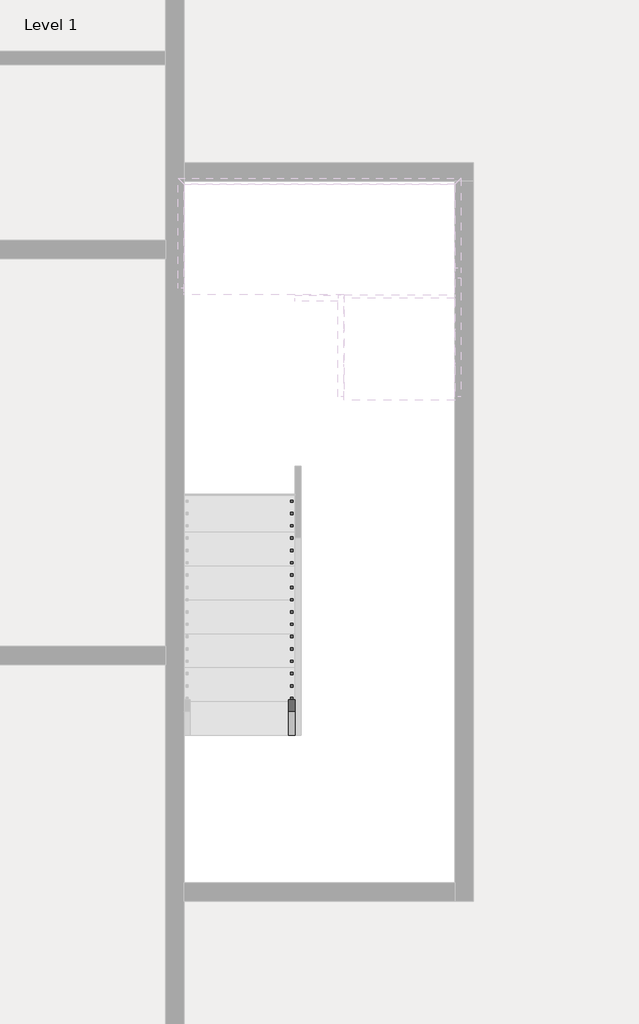
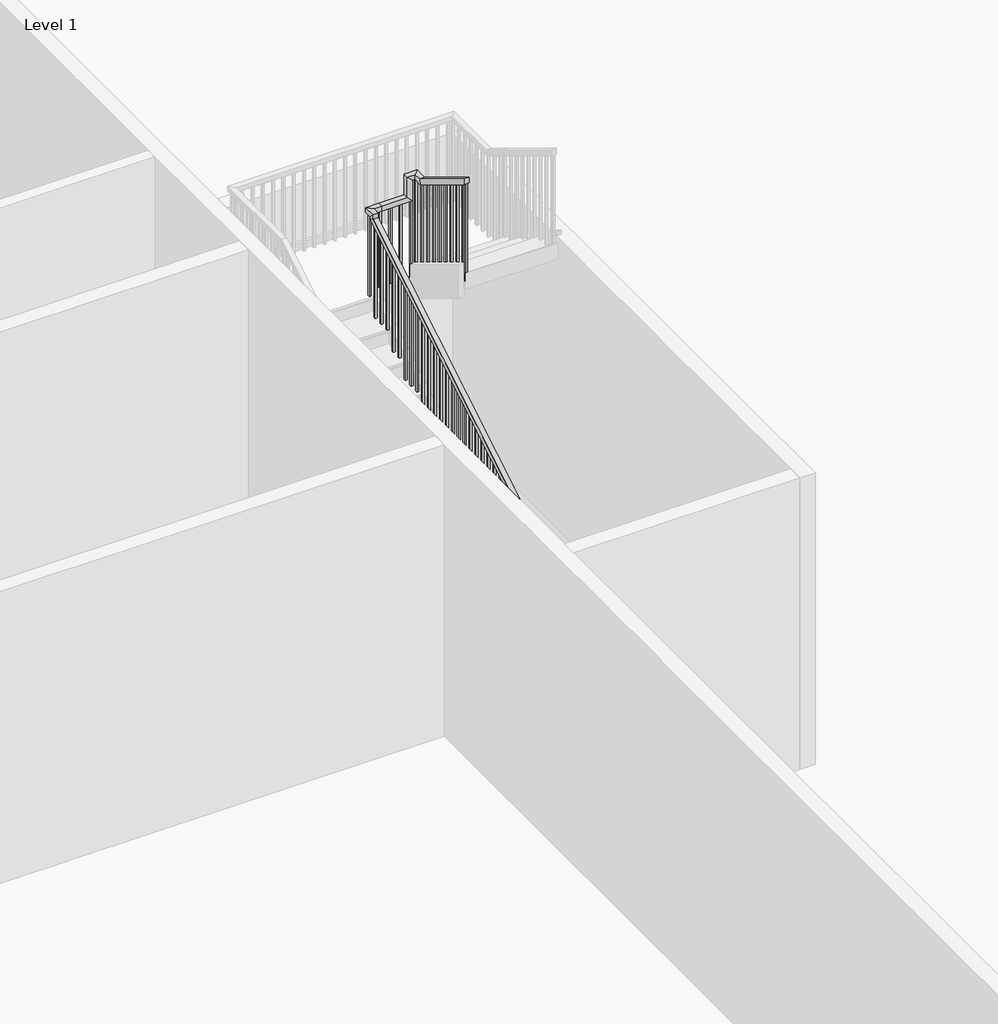
# One storey, part 5 of 8: 1 railing.
"""IFC4 building model written with IfcOpenShell, lengths in millimetres."""

from ifc_helpers import new_model, si_unit, frame, origin, place, context, project, spatial, polyline, outline, extrude, faceted_brep, element, save

model = new_model("IFC4")

# Units and contexts
model_context = context("Model", 3, world=origin())
ifc_project = project(units=[si_unit("LENGTHUNIT", "METRE", prefix="MILLI")], contexts=[model_context])

# Site, building, storey
site = spatial("IfcSite", under=ifc_project)
building = spatial("IfcBuilding", under=site)
storey = spatial("IfcBuildingStorey", under=building, Name="Level 1", Elevation=25234.6172466)

# Railing
placement = place(None, origin())
element("IfcRailing", 1, ObjectType="Handrail - Rectangular", at=placement, inside=storey, context=model_context, shape_type="SolidModel", body=[
    faceted_brep([(-2753.8415084, -23154.3851539, 26318.3505799), (-2753.8415084, -23154.3851539, 26258.9491197), (-2703.0415084, -23154.3851539, 26258.9491197), (-2703.0415084, -23154.3851539, 26318.3505799), (-2753.8415084, -19598.3851539, 28473.5020951), (-2753.8415084, -19547.5851539, 28444.8885136), (-2703.0415084, -19547.5851539, 28444.8885136), (-2703.0415084, -19598.3851539, 28473.5020951), (-2753.8415084, -19598.3851539, 28519.6839133), (-2753.8415084, -19547.5851539, 28468.8839133), (-2703.0415084, -19547.5851539, 28468.8839133), (-2703.0415084, -19598.3851539, 28519.6839133), (-2753.8415084, -19471.3851539, 28519.6839133), (-2753.8415084, -19471.3851539, 28468.8839133), (-2703.0415084, -19522.1851539, 28468.8839133), (-2703.0415084, -19522.1851539, 28519.6839133), (-2626.8415084, -19471.3851539, 28519.6839133), (-2626.8415084, -19471.3851539, 28468.8839133), (-2626.8415084, -19522.1851539, 28468.8839133), (-2626.8415084, -19522.1851539, 28519.6839133), (-2372.8415084, -19471.3851539, 28519.6839133), (-2322.0415084, -19471.3851539, 28468.8839133), (-2322.0415084, -19522.1851539, 28468.8839133), (-2372.8415084, -19522.1851539, 28519.6839133), (-2372.8415084, -19471.3851539, 28735.1990648), (-2322.0415084, -19471.3851539, 28684.3990648), (-2322.0415084, -19522.1851539, 28684.3990648), (-2372.8415084, -19522.1851539, 28735.1990648), (-2245.8415084, -19471.3851539, 28735.1990648), (-2245.8415084, -19471.3851539, 28684.3990648), (-2296.6415084, -19522.1851539, 28684.3990648), (-2296.6415084, -19522.1851539, 28735.1990648), (-2245.8415084, -19598.3851539, 28735.1990648), (-2245.8415084, -19612.5775633, 28684.3990648), (-2296.6415084, -19612.5775633, 28684.3990648), (-2296.6415084, -19598.3851539, 28735.1990648), (-2245.8415084, -20360.3851539, 29197.0172466), (-2296.6415084, -20360.3851539, 29197.0172466), (-2296.6415084, -20360.3851539, 29137.6157863), (-2245.8415084, -20360.3851539, 29137.6157863)], [[[0, 1, 2, 3]], [[1, 0, 4, 5]], [[2, 1, 5, 6]], [[3, 2, 6, 7]], [[0, 3, 7, 4]], [[5, 4, 8, 9]], [[6, 5, 9, 10]], [[7, 6, 10, 11]], [[4, 7, 11, 8]], [[9, 8, 12, 13]], [[10, 9, 13, 14]], [[11, 10, 14, 15]], [[8, 11, 15, 12]], [[13, 12, 16, 17]], [[14, 13, 17, 18]], [[15, 14, 18, 19]], [[12, 15, 19, 16]], [[17, 16, 20, 21]], [[18, 17, 21, 22]], [[19, 18, 22, 23]], [[16, 19, 23, 20]], [[21, 20, 24, 25]], [[22, 21, 25, 26]], [[23, 22, 26, 27]], [[20, 23, 27, 24]], [[25, 24, 28, 29]], [[26, 25, 29, 30]], [[27, 26, 30, 31]], [[24, 27, 31, 28]], [[29, 28, 32, 33]], [[30, 29, 33, 34]], [[31, 30, 34, 35]], [[28, 31, 35, 32]], [[36, 37, 38, 39]], [[33, 32, 36, 39]], [[34, 33, 39, 38]], [[35, 34, 38, 37]], [[32, 35, 37, 36]]]),
    extrude(outline(polyline([(-20319.1101539, 29112.6006348), (-20300.0601539, 29101.0551803), (-20300.0601539, 28113.2839133), (-20319.1101539, 28113.2839133), (-20319.1101539, 29112.6006348)])), frame((-2280.7665084, 0.0, 0.0), z_axis=(1.0, 0.0, 0.0), x_axis=(0.0, 1.0, 0.0)), (0.0, 0.0, 1.0), 19.05),
    extrude(outline(polyline([(-20217.5101539, 29051.0248773), (-20198.4601539, 29039.4794227), (-20198.4601539, 28113.2839133), (-20217.5101539, 28113.2839133), (-20217.5101539, 29051.0248773)])), frame((-2280.7665084, 0.0, 0.0), z_axis=(1.0, 0.0, 0.0), x_axis=(0.0, 1.0, 0.0)), (0.0, 0.0, 1.0), 19.05),
    extrude(outline(polyline([(-20115.9101539, 28989.4491197), (-20096.8601539, 28977.9036651), (-20096.8601539, 28113.2839133), (-20115.9101539, 28113.2839133), (-20115.9101539, 28989.4491197)])), frame((-2280.7665084, 0.0, 0.0), z_axis=(1.0, 0.0, 0.0), x_axis=(0.0, 1.0, 0.0)), (0.0, 0.0, 1.0), 19.05),
    extrude(outline(polyline([(-20014.3101539, 28927.8733621), (-19995.2601539, 28916.3279076), (-19995.2601539, 27943.9505799), (-20014.3101539, 27943.9505799), (-20014.3101539, 28927.8733621)])), frame((-2280.7665084, 0.0, 0.0), z_axis=(1.0, 0.0, 0.0), x_axis=(0.0, 1.0, 0.0)), (0.0, 0.0, 1.0), 19.05),
    extrude(outline(polyline([(-19912.7101539, 28866.2976045), (-19893.6601539, 28854.75215), (-19893.6601539, 27943.9505799), (-19912.7101539, 27943.9505799), (-19912.7101539, 28866.2976045)])), frame((-2280.7665084, 0.0, 0.0), z_axis=(1.0, 0.0, 0.0), x_axis=(0.0, 1.0, 0.0)), (0.0, 0.0, 1.0), 19.05),
    extrude(outline(polyline([(-19811.1101539, 28804.721847), (-19792.0601539, 28793.1763924), (-19792.0601539, 27943.9505799), (-19811.1101539, 27943.9505799), (-19811.1101539, 28804.721847)])), frame((-2280.7665084, 0.0, 0.0), z_axis=(1.0, 0.0, 0.0), x_axis=(0.0, 1.0, 0.0)), (0.0, 0.0, 1.0), 19.05),
    extrude(outline(polyline([(-19709.5101539, 28743.1460894), (-19690.4601539, 28731.6006348), (-19690.4601539, 27774.6172466), (-19709.5101539, 27774.6172466), (-19709.5101539, 28743.1460894)])), frame((-2280.7665084, 0.0, 0.0), z_axis=(1.0, 0.0, 0.0), x_axis=(0.0, 1.0, 0.0)), (0.0, 0.0, 1.0), 19.05),
    extrude(outline(polyline([(-19607.9101539, 28681.5703318), (-19588.8601539, 28670.0248773), (-19588.8601539, 27774.6172466), (-19607.9101539, 27774.6172466), (-19607.9101539, 28681.5703318)])), frame((-2280.7665084, 0.0, 0.0), z_axis=(1.0, 0.0, 0.0), x_axis=(0.0, 1.0, 0.0)), (0.0, 0.0, 1.0), 19.05),
    extrude(outline(polyline([(-2331.5665084, -19506.3101539), (-2331.5665084, -19487.2601539), (-2312.5165084, -19487.2601539), (-2312.5165084, -19506.3101539), (-2331.5665084, -19506.3101539)])), frame((0.0, 0.0, 27605.2839133), z_axis=(0.0, 0.0, 1.0), x_axis=(1.0, 0.0, 0.0)), (0.0, 0.0, 1.0), 1079.1151515),
    extrude(outline(polyline([(-2433.1665084, -19506.3101539), (-2433.1665084, -19487.2601539), (-2414.1165084, -19487.2601539), (-2414.1165084, -19506.3101539), (-2433.1665084, -19506.3101539)])), frame((0.0, 0.0, 27605.2839133), z_axis=(0.0, 0.0, 1.0), x_axis=(1.0, 0.0, 0.0)), (0.0, 0.0, 1.0), 863.6),
    extrude(outline(polyline([(-2534.7665084, -19506.3101539), (-2534.7665084, -19487.2601539), (-2515.7165084, -19487.2601539), (-2515.7165084, -19506.3101539), (-2534.7665084, -19506.3101539)])), frame((0.0, 0.0, 27605.2839133), z_axis=(0.0, 0.0, 1.0), x_axis=(1.0, 0.0, 0.0)), (0.0, 0.0, 1.0), 863.6),
    extrude(outline(polyline([(-2636.3665084, -19506.3101539), (-2636.3665084, -19487.2601539), (-2617.3165084, -19487.2601539), (-2617.3165084, -19506.3101539), (-2636.3665084, -19506.3101539)])), frame((0.0, 0.0, 27605.2839133), z_axis=(0.0, 0.0, 1.0), x_axis=(1.0, 0.0, 0.0)), (0.0, 0.0, 1.0), 863.6),
    extrude(outline(polyline([(-19607.9101539, 28408.3279076), (-19588.8601539, 28419.8733621), (-19588.8601539, 27435.9505799), (-19607.9101539, 27435.9505799), (-19607.9101539, 28408.3279076)])), frame((-2737.9665084, 0.0, 0.0), z_axis=(1.0, 0.0, 0.0), x_axis=(0.0, 1.0, 0.0)), (0.0, 0.0, 1.0), 19.05),
    extrude(outline(polyline([(-19709.5101539, 28346.75215), (-19690.4601539, 28358.2976045), (-19690.4601539, 27435.9505799), (-19709.5101539, 27435.9505799), (-19709.5101539, 28346.75215)])), frame((-2737.9665084, 0.0, 0.0), z_axis=(1.0, 0.0, 0.0), x_axis=(0.0, 1.0, 0.0)), (0.0, 0.0, 1.0), 19.05),
    extrude(outline(polyline([(-19811.1101539, 28285.1763924), (-19792.0601539, 28296.721847), (-19792.0601539, 27435.9505799), (-19811.1101539, 27435.9505799), (-19811.1101539, 28285.1763924)])), frame((-2737.9665084, 0.0, 0.0), z_axis=(1.0, 0.0, 0.0), x_axis=(0.0, 1.0, 0.0)), (0.0, 0.0, 1.0), 19.05),
    extrude(outline(polyline([(-19912.7101539, 28223.6006348), (-19893.6601539, 28235.1460894), (-19893.6601539, 27266.6172466), (-19912.7101539, 27266.6172466), (-19912.7101539, 28223.6006348)])), frame((-2737.9665084, 0.0, 0.0), z_axis=(1.0, 0.0, 0.0), x_axis=(0.0, 1.0, 0.0)), (0.0, 0.0, 1.0), 19.05),
    extrude(outline(polyline([(-20014.3101539, 28162.0248773), (-19995.2601539, 28173.5703318), (-19995.2601539, 27266.6172466), (-20014.3101539, 27266.6172466), (-20014.3101539, 28162.0248773)])), frame((-2737.9665084, 0.0, 0.0), z_axis=(1.0, 0.0, 0.0), x_axis=(0.0, 1.0, 0.0)), (0.0, 0.0, 1.0), 19.05),
    extrude(outline(polyline([(-20115.9101539, 28100.4491197), (-20096.8601539, 28111.9945742), (-20096.8601539, 27097.2839133), (-20115.9101539, 27097.2839133), (-20115.9101539, 28100.4491197)])), frame((-2737.9665084, 0.0, 0.0), z_axis=(1.0, 0.0, 0.0), x_axis=(0.0, 1.0, 0.0)), (0.0, 0.0, 1.0), 19.05),
    extrude(outline(polyline([(-20217.5101539, 28038.8733621), (-20198.4601539, 28050.4188167), (-20198.4601539, 27097.2839133), (-20217.5101539, 27097.2839133), (-20217.5101539, 28038.8733621)])), frame((-2737.9665084, 0.0, 0.0), z_axis=(1.0, 0.0, 0.0), x_axis=(0.0, 1.0, 0.0)), (0.0, 0.0, 1.0), 19.05),
    extrude(outline(polyline([(-20319.1101539, 27977.2976045), (-20300.0601539, 27988.8430591), (-20300.0601539, 27097.2839133), (-20319.1101539, 27097.2839133), (-20319.1101539, 27977.2976045)])), frame((-2737.9665084, 0.0, 0.0), z_axis=(1.0, 0.0, 0.0), x_axis=(0.0, 1.0, 0.0)), (0.0, 0.0, 1.0), 19.05),
    extrude(outline(polyline([(-20420.7101539, 27915.721847), (-20401.6601539, 27927.2673015), (-20401.6601539, 26927.9505799), (-20420.7101539, 26927.9505799), (-20420.7101539, 27915.721847)])), frame((-2737.9665084, 0.0, 0.0), z_axis=(1.0, 0.0, 0.0), x_axis=(0.0, 1.0, 0.0)), (0.0, 0.0, 1.0), 19.05),
    extrude(outline(polyline([(-20522.3101539, 27854.1460894), (-20503.2601539, 27865.6915439), (-20503.2601539, 26927.9505799), (-20522.3101539, 26927.9505799), (-20522.3101539, 27854.1460894)])), frame((-2737.9665084, 0.0, 0.0), z_axis=(1.0, 0.0, 0.0), x_axis=(0.0, 1.0, 0.0)), (0.0, 0.0, 1.0), 19.05),
    extrude(outline(polyline([(-20623.9101539, 27792.5703318), (-20604.8601539, 27804.1157863), (-20604.8601539, 26927.9505799), (-20623.9101539, 26927.9505799), (-20623.9101539, 27792.5703318)])), frame((-2737.9665084, 0.0, 0.0), z_axis=(1.0, 0.0, 0.0), x_axis=(0.0, 1.0, 0.0)), (0.0, 0.0, 1.0), 19.05),
    extrude(outline(polyline([(-20725.5101539, 27730.9945742), (-20706.4601539, 27742.5400288), (-20706.4601539, 26758.6172466), (-20725.5101539, 26758.6172466), (-20725.5101539, 27730.9945742)])), frame((-2737.9665084, 0.0, 0.0), z_axis=(1.0, 0.0, 0.0), x_axis=(0.0, 1.0, 0.0)), (0.0, 0.0, 1.0), 19.05),
    extrude(outline(polyline([(-20827.1101539, 27669.4188167), (-20808.0601539, 27680.9642712), (-20808.0601539, 26758.6172466), (-20827.1101539, 26758.6172466), (-20827.1101539, 27669.4188167)])), frame((-2737.9665084, 0.0, 0.0), z_axis=(1.0, 0.0, 0.0), x_axis=(0.0, 1.0, 0.0)), (0.0, 0.0, 1.0), 19.05),
    extrude(outline(polyline([(-20928.7101539, 27607.8430591), (-20909.6601539, 27619.3885136), (-20909.6601539, 26758.6172466), (-20928.7101539, 26758.6172466), (-20928.7101539, 27607.8430591)])), frame((-2737.9665084, 0.0, 0.0), z_axis=(1.0, 0.0, 0.0), x_axis=(0.0, 1.0, 0.0)), (0.0, 0.0, 1.0), 19.05),
    extrude(outline(polyline([(-21030.3101539, 27546.2673015), (-21011.2601539, 27557.812756), (-21011.2601539, 26589.2839133), (-21030.3101539, 26589.2839133), (-21030.3101539, 27546.2673015)])), frame((-2737.9665084, 0.0, 0.0), z_axis=(1.0, 0.0, 0.0), x_axis=(0.0, 1.0, 0.0)), (0.0, 0.0, 1.0), 19.05),
    extrude(outline(polyline([(-21131.9101539, 27484.6915439), (-21112.8601539, 27496.2369985), (-21112.8601539, 26589.2839133), (-21131.9101539, 26589.2839133), (-21131.9101539, 27484.6915439)])), frame((-2737.9665084, 0.0, 0.0), z_axis=(1.0, 0.0, 0.0), x_axis=(0.0, 1.0, 0.0)), (0.0, 0.0, 1.0), 19.05),
    extrude(outline(polyline([(-21233.5101539, 27423.1157863), (-21214.4601539, 27434.6612409), (-21214.4601539, 26419.9505799), (-21233.5101539, 26419.9505799), (-21233.5101539, 27423.1157863)])), frame((-2737.9665084, 0.0, 0.0), z_axis=(1.0, 0.0, 0.0), x_axis=(0.0, 1.0, 0.0)), (0.0, 0.0, 1.0), 19.05),
    extrude(outline(polyline([(-21335.1101539, 27361.5400288), (-21316.0601539, 27373.0854833), (-21316.0601539, 26419.9505799), (-21335.1101539, 26419.9505799), (-21335.1101539, 27361.5400288)])), frame((-2737.9665084, 0.0, 0.0), z_axis=(1.0, 0.0, 0.0), x_axis=(0.0, 1.0, 0.0)), (0.0, 0.0, 1.0), 19.05),
    extrude(outline(polyline([(-21436.7101539, 27299.9642712), (-21417.6601539, 27311.5097257), (-21417.6601539, 26419.9505799), (-21436.7101539, 26419.9505799), (-21436.7101539, 27299.9642712)])), frame((-2737.9665084, 0.0, 0.0), z_axis=(1.0, 0.0, 0.0), x_axis=(0.0, 1.0, 0.0)), (0.0, 0.0, 1.0), 19.05),
    extrude(outline(polyline([(-21538.3101539, 27238.3885136), (-21519.2601539, 27249.9339682), (-21519.2601539, 26250.6172466), (-21538.3101539, 26250.6172466), (-21538.3101539, 27238.3885136)])), frame((-2737.9665084, 0.0, 0.0), z_axis=(1.0, 0.0, 0.0), x_axis=(0.0, 1.0, 0.0)), (0.0, 0.0, 1.0), 19.05),
    extrude(outline(polyline([(-21639.9101539, 27176.812756), (-21620.8601539, 27188.3582106), (-21620.8601539, 26250.6172466), (-21639.9101539, 26250.6172466), (-21639.9101539, 27176.812756)])), frame((-2737.9665084, 0.0, 0.0), z_axis=(1.0, 0.0, 0.0), x_axis=(0.0, 1.0, 0.0)), (0.0, 0.0, 1.0), 19.05),
    extrude(outline(polyline([(-21741.5101539, 27115.2369985), (-21722.4601539, 27126.782453), (-21722.4601539, 26250.6172466), (-21741.5101539, 26250.6172466), (-21741.5101539, 27115.2369985)])), frame((-2737.9665084, 0.0, 0.0), z_axis=(1.0, 0.0, 0.0), x_axis=(0.0, 1.0, 0.0)), (0.0, 0.0, 1.0), 19.05),
    extrude(outline(polyline([(-21843.1101539, 27053.6612409), (-21824.0601539, 27065.2066954), (-21824.0601539, 26081.2839133), (-21843.1101539, 26081.2839133), (-21843.1101539, 27053.6612409)])), frame((-2737.9665084, 0.0, 0.0), z_axis=(1.0, 0.0, 0.0), x_axis=(0.0, 1.0, 0.0)), (0.0, 0.0, 1.0), 19.05),
    extrude(outline(polyline([(-21944.7101539, 26992.0854833), (-21925.6601539, 27003.6309379), (-21925.6601539, 26081.2839133), (-21944.7101539, 26081.2839133), (-21944.7101539, 26992.0854833)])), frame((-2737.9665084, 0.0, 0.0), z_axis=(1.0, 0.0, 0.0), x_axis=(0.0, 1.0, 0.0)), (0.0, 0.0, 1.0), 19.05),
    extrude(outline(polyline([(-22046.3101539, 26930.5097257), (-22027.2601539, 26942.0551803), (-22027.2601539, 26081.2839133), (-22046.3101539, 26081.2839133), (-22046.3101539, 26930.5097257)])), frame((-2737.9665084, 0.0, 0.0), z_axis=(1.0, 0.0, 0.0), x_axis=(0.0, 1.0, 0.0)), (0.0, 0.0, 1.0), 19.05),
    extrude(outline(polyline([(-22147.9101539, 26868.9339682), (-22128.8601539, 26880.4794227), (-22128.8601539, 25911.9505799), (-22147.9101539, 25911.9505799), (-22147.9101539, 26868.9339682)])), frame((-2737.9665084, 0.0, 0.0), z_axis=(1.0, 0.0, 0.0), x_axis=(0.0, 1.0, 0.0)), (0.0, 0.0, 1.0), 19.05),
    extrude(outline(polyline([(-22249.5101539, 26807.3582106), (-22230.4601539, 26818.9036651), (-22230.4601539, 25911.9505799), (-22249.5101539, 25911.9505799), (-22249.5101539, 26807.3582106)])), frame((-2737.9665084, 0.0, 0.0), z_axis=(1.0, 0.0, 0.0), x_axis=(0.0, 1.0, 0.0)), (0.0, 0.0, 1.0), 19.05),
    extrude(outline(polyline([(-22351.1101539, 26745.782453), (-22332.0601539, 26757.3279076), (-22332.0601539, 25742.6172466), (-22351.1101539, 25742.6172466), (-22351.1101539, 26745.782453)])), frame((-2737.9665084, 0.0, 0.0), z_axis=(1.0, 0.0, 0.0), x_axis=(0.0, 1.0, 0.0)), (0.0, 0.0, 1.0), 19.05),
    extrude(outline(polyline([(-22452.7101539, 26684.2066954), (-22433.6601539, 26695.75215), (-22433.6601539, 25742.6172466), (-22452.7101539, 25742.6172466), (-22452.7101539, 26684.2066954)])), frame((-2737.9665084, 0.0, 0.0), z_axis=(1.0, 0.0, 0.0), x_axis=(0.0, 1.0, 0.0)), (0.0, 0.0, 1.0), 19.05),
    extrude(outline(polyline([(-22554.3101539, 26622.6309379), (-22535.2601539, 26634.1763924), (-22535.2601539, 25742.6172466), (-22554.3101539, 25742.6172466), (-22554.3101539, 26622.6309379)])), frame((-2737.9665084, 0.0, 0.0), z_axis=(1.0, 0.0, 0.0), x_axis=(0.0, 1.0, 0.0)), (0.0, 0.0, 1.0), 19.05),
    extrude(outline(polyline([(-22655.9101539, 26561.0551803), (-22636.8601539, 26572.6006348), (-22636.8601539, 25573.2839133), (-22655.9101539, 25573.2839133), (-22655.9101539, 26561.0551803)])), frame((-2737.9665084, 0.0, 0.0), z_axis=(1.0, 0.0, 0.0), x_axis=(0.0, 1.0, 0.0)), (0.0, 0.0, 1.0), 19.05),
    extrude(outline(polyline([(-22757.5101539, 26499.4794227), (-22738.4601539, 26511.0248773), (-22738.4601539, 25573.2839133), (-22757.5101539, 25573.2839133), (-22757.5101539, 26499.4794227)])), frame((-2737.9665084, 0.0, 0.0), z_axis=(1.0, 0.0, 0.0), x_axis=(0.0, 1.0, 0.0)), (0.0, 0.0, 1.0), 19.05),
    extrude(outline(polyline([(-22859.1101539, 26437.9036651), (-22840.0601539, 26449.4491197), (-22840.0601539, 25573.2839133), (-22859.1101539, 25573.2839133), (-22859.1101539, 26437.9036651)])), frame((-2737.9665084, 0.0, 0.0), z_axis=(1.0, 0.0, 0.0), x_axis=(0.0, 1.0, 0.0)), (0.0, 0.0, 1.0), 19.05),
    extrude(outline(polyline([(-22960.7101539, 26376.3279076), (-22941.6601539, 26387.8733621), (-22941.6601539, 25403.9505799), (-22960.7101539, 25403.9505799), (-22960.7101539, 26376.3279076)])), frame((-2737.9665084, 0.0, 0.0), z_axis=(1.0, 0.0, 0.0), x_axis=(0.0, 1.0, 0.0)), (0.0, 0.0, 1.0), 19.05),
    extrude(outline(polyline([(-23062.3101539, 26314.75215), (-23043.2601539, 26326.2976045), (-23043.2601539, 25403.9505799), (-23062.3101539, 25403.9505799), (-23062.3101539, 26314.75215)])), frame((-2737.9665084, 0.0, 0.0), z_axis=(1.0, 0.0, 0.0), x_axis=(0.0, 1.0, 0.0)), (0.0, 0.0, 1.0), 19.05),
    extrude(outline(polyline([(-2280.7665084, -19506.3101539), (-2280.7665084, -19487.2601539), (-2261.7165084, -19487.2601539), (-2261.7165084, -19506.3101539), (-2280.7665084, -19506.3101539)])), frame((0.0, 0.0, 27605.2839133), z_axis=(0.0, 0.0, 1.0), x_axis=(1.0, 0.0, 0.0)), (0.0, 0.0, 1.0), 1079.1151515),
    extrude(outline(polyline([(-2718.9165084, -19506.3101539), (-2737.9665084, -19506.3101539), (-2737.9665084, -19487.2601539), (-2718.9165084, -19487.2601539), (-2718.9165084, -19506.3101539)])), frame((0.0, 0.0, 27605.2839133), z_axis=(0.0, 0.0, 1.0), x_axis=(1.0, 0.0, 0.0)), (0.0, 0.0, 1.0), 863.6),
    extrude(outline(polyline([(-20360.3851539, 29137.6157863), (-20341.3351539, 29126.0703318), (-20341.3351539, 28113.2839133), (-20360.3851539, 28113.2839133), (-20360.3851539, 29137.6157863)])), frame((-2280.7665084, 0.0, 0.0), z_axis=(1.0, 0.0, 0.0), x_axis=(0.0, 1.0, 0.0)), (0.0, 0.0, 1.0), 19.05),
    extrude(outline(polyline([(-23154.3851539, 26258.9491197), (-23135.3351539, 26270.4945742), (-23135.3351539, 25403.9505799), (-23154.3851539, 25403.9505799), (-23154.3851539, 26258.9491197)])), frame((-2737.9665084, 0.0, 0.0), z_axis=(1.0, 0.0, 0.0), x_axis=(0.0, 1.0, 0.0)), (0.0, 0.0, 1.0), 19.05),
])

save(model, "model.ifc")

# Revit data of these elements
# Type "Handrail - Rectangular"
#   Assembly Code = "C2010400"
#   built-in parameter 1008612 = 0.0416667 (stored number, unit not read)
#   built-in parameter 1008611 = 0.0416667 (stored number, unit not read)
#   built-in parameter 1008609 = 0.333333 (stored number, unit not read)
#   built-in parameter 1008604 = 0.166667 (stored number, unit not read)
#   built-in parameter 1008603 = 0.166667 (stored number, unit not read)
#   Railing Height = 3' - 0"
#   built-in parameter 1008630 = 2
#   built-in parameter 1008610 = 2
#   built-in parameter 1008618 = Baluster - Square : 3/4"
# Element 1 (IfcRailing, "Handrail - Rectangular")
#   Phase Created = New Construction
